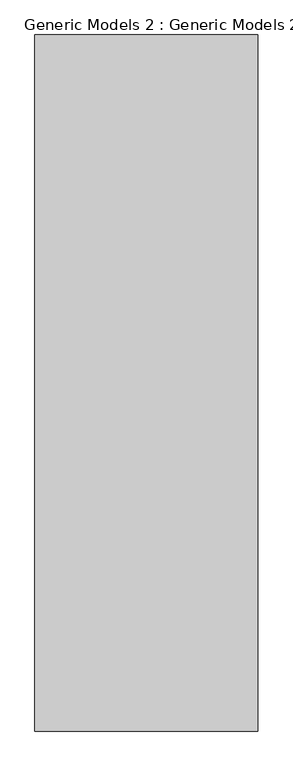
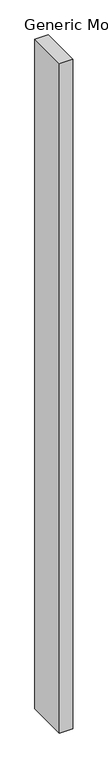
"""IFC4 building model written with IfcOpenShell, lengths in millimetres: proxy geometry, Generic Models 2 : Generic Models 2."""

from ifc_helpers import new_model, si_unit, origin, origin_with_axes, place, context, project, spatial, polyline, outline, extrude, source, transform, mapped, element, save


def generic_models_2_generic_models_2_24f987b9(model_context):
    return source(origin(), model_context, "Body", "SweptSolid", [
        extrude(outline(polyline([(-3801.1300045, -16327.2030397), (-4957.034663, -16327.2030397), (-4957.034663, -12718.8007309), (-3801.1300045, -12718.8007309), (-3801.1300045, -16327.2030397)])), origin_with_axes(), (0.0, 0.0, 1.0), 60271.827178),
    ])


if __name__ == "__main__":
    model = new_model("IFC4")
    model_context = context("Model", 3, world=origin())
    ifc_project = project(units=[si_unit("LENGTHUNIT", "METRE", prefix="MILLI")], contexts=[model_context])
    site = spatial("IfcSite", under=ifc_project)
    building = spatial("IfcBuilding", under=site)
    placement = place(None, origin())
    generic_models_2_generic_models_2_shape = generic_models_2_generic_models_2_24f987b9(model_context)
    element("IfcBuildingElementProxy", 1, Name="Generic Models 2 : Generic Models 2", ObjectType="Generic Models 2 : Generic Models 2", at=placement, inside=building, context=model_context, shape_type="MappedRepresentation", body=[
        mapped(generic_models_2_generic_models_2_shape, transform((0.0, 0.0, 0.0), x_axis=(1.0, 0.0, 0.0), y_axis=(0.0, 1.0, 0.0), z_axis=(0.0, 0.0, 1.0))),
    ])
    save(model, "model.ifc")
